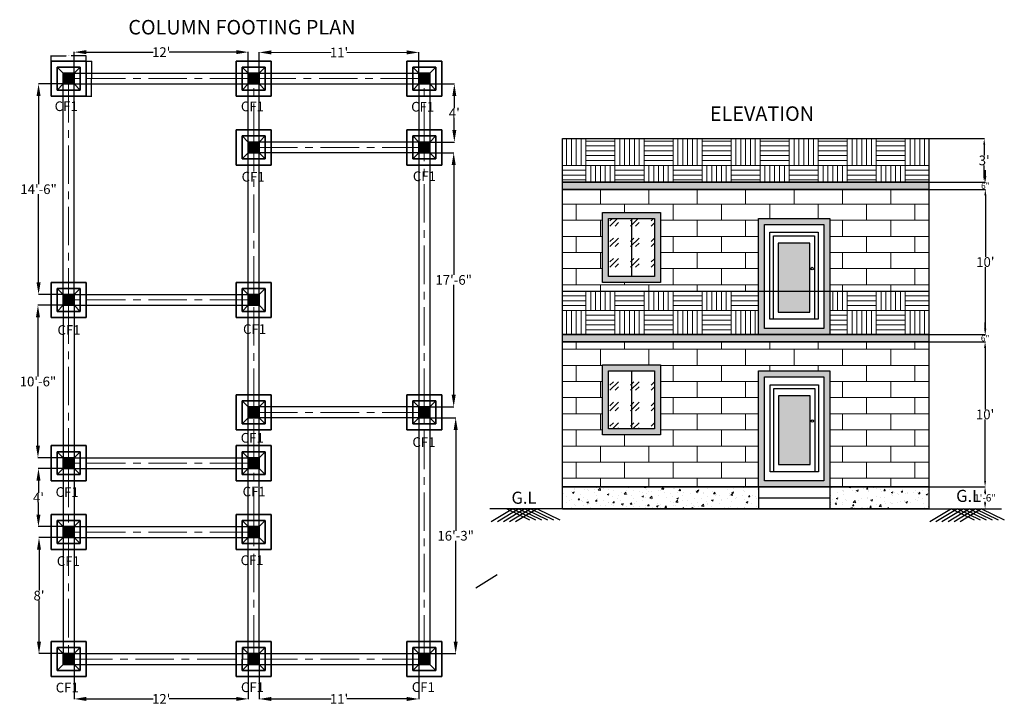
# Model space of a CAD drawing. Units: inches. Extents: x -25 to 789, y -921 to 230.
# Tile 1 of 5: x -25 to 789, y -921 to -354. Entities that reach past the tile are written whole.
import ezdxf

# ---------------------------------------------------------------- set-up
doc = ezdxf.new("R2010")
doc.units = ezdxf.units.IN
doc.header["$MEASUREMENT"] = 0
doc.linetypes.add('CENTER', pattern=[50.8, 31.75, -6.35, 6.35, -6.35])
for name, color, linetype, lineweight in [('A-ANNO-DIMS', 2, 'Continuous', 18), ('A-ANNO-TEXT', 7, 'Continuous', 18), ('A-DOOR', 4, 'Continuous', 25), ('A-ELEV', 7, 'Continuous', 25), ('A-ELEV-PATT', 252, 'Continuous', 13), ('S-ANNO-DIMS', 2, 'Continuous', 18), ('S-ANNO-TEXT', 7, 'Continuous', 18), ('S-BEAM', 4, 'Continuous', 25), ('S-FNDN', 2, 'Continuous', 35), ('S-FNDN-PATT', 8, 'Continuous', 13), ('S-GRID', 6, 'CENTER', 18)]:
    doc.layers.add(name, color=color, linetype=linetype, lineweight=lineweight)
doc.styles.get("Standard").update_dxf_attribs({"font": 'arial.ttf'})
doc.dimstyles.get("Standard").update_dxf_attribs({"dimtxt": 0.18, "dimasz": 0.18, "dimexe": 0.18, "dimexo": 0.0625, "dimgap": 0.09, "dimtad": 0, "dimtih": 1, "dimtoh": 1, "dimdec": 1, "dimzin": 0, "dimdsep": 46, "dimlunit": 4, "dimtxsty": 'Standard', "dimcen": 0.09, "dimadec": 0, "dimazin": 0, "dimtfac": 1, "dimtdec": 1, "dimtofl": 0, "dimtmove": 0, "dimatfit": 3, "dimfxl": 1, "dimtolj": 1, "dimtzin": 0, "dimarcsym": 0})

# ---------------------------------------------------------------- blocks, each defined once
blk = doc.blocks.new('*U29')
blk.add_lwpolyline([(3.12, 0.01), (0.12, 0.01), (0.12, 72.01), (40.12, 72.01), (40.12, 0.01), (37.12, 0.01)])
for points in [[(37.12, 68.99), (37.12, 0.01), (3.12, 0.01), (3.12, 68.99)], [(33.12, 6.01), (33.12, 62.99), (7.12, 62.99), (7.12, 6.01)]]:
    blk.add_lwpolyline(points, close=True)
blk.add_circle((35.12, 42.01), 1)
blk = doc.blocks.new('*D30')
at = {"layer": 'A-ANNO-DIMS', "color": 0, "lineweight": -2, "transparency": 16777216}
for p, q in [((773.58, -483.04), (773.58, -478.04)), ((727.04, -488.04), (773.76, -488.04)), ((727.04, -494.04), (773.76, -494.04)), ((773.58, -499.04), (773.58, -504.04))]:
    blk.add_line(p, q, dxfattribs=at)
at = {"layer": 'A-ANNO-DIMS', "color": 0, "transparency": 16777216}
for points in [[(772.75, -483.04), (774.42, -483.04), (773.58, -488.04)], [(772.75, -499.04), (774.42, -499.04), (773.58, -494.04)]]:
    blk.add_solid(points, dxfattribs=at)
at = {"layer": 'Defpoints', "color": 0, "transparency": 16777216}
for p in [(726.98, -488.04), (773.58, -488.04), (726.98, -494.04)]:
    blk.add_point(p, dxfattribs=at)
at = {"layer": 'A-ANNO-DIMS', "color": 0, "transparency": 16777216, "insert": (773.58, -491.04), "char_height": 5, "attachment_point": 5}
blk.add_mtext('\\A1;6"', dxfattribs=at)
blk = doc.blocks.new('*D31')
at = {"layer": 'A-ANNO-DIMS', "color": 0, "lineweight": -2, "transparency": 16777216}
for p, q in [((727.04, -452.04), (772.82, -452.04)), ((772.64, -457.04), (772.64, -465.87)), ((772.64, -483.04), (772.64, -474.22)), ((727.04, -488.04), (772.82, -488.04))]:
    blk.add_line(p, q, dxfattribs=at)
at = {"layer": 'A-ANNO-DIMS', "color": 0, "transparency": 16777216}
for points in [[(771.81, -457.04), (773.48, -457.04), (772.64, -452.04)], [(771.81, -483.04), (773.48, -483.04), (772.64, -488.04)]]:
    blk.add_solid(points, dxfattribs=at)
at = {"layer": 'Defpoints', "color": 0, "transparency": 16777216}
for p in [(726.98, -452.04), (772.64, -452.04), (726.98, -488.04)]:
    blk.add_point(p, dxfattribs=at)
at = {"layer": 'A-ANNO-DIMS', "color": 0, "transparency": 16777216, "insert": (772.64, -470.04), "char_height": 8, "attachment_point": 5}
blk.add_mtext("\\A1;3'", dxfattribs=at)
blk = doc.blocks.new('*D32')
at = {"layer": 'A-ANNO-DIMS', "color": 0, "lineweight": -2, "transparency": 16777216}
for p, q in [((727.04, -740.04), (773.55, -740.04)), ((773.37, -745.04), (773.37, -745.89)), ((773.37, -753.04), (773.37, -752.2)), ((727.04, -758.04), (773.55, -758.04))]:
    blk.add_line(p, q, dxfattribs=at)
at = {"layer": 'A-ANNO-DIMS', "color": 0, "transparency": 16777216}
for points in [[(772.53, -745.04), (774.2, -745.04), (773.37, -740.04)], [(772.53, -753.04), (774.2, -753.04), (773.37, -758.04)]]:
    blk.add_solid(points, dxfattribs=at)
at = {"layer": 'Defpoints', "color": 0, "transparency": 16777216}
for p in [(726.98, -740.04), (773.37, -740.04), (726.98, -758.04)]:
    blk.add_point(p, dxfattribs=at)
at = {"layer": 'A-ANNO-DIMS', "color": 0, "transparency": 16777216, "insert": (773.37, -749.04), "char_height": 6, "attachment_point": 5}
blk.add_mtext('\\A1;1\'-6"', dxfattribs=at)
blk = doc.blocks.new('*D33')
at = {"layer": 'A-ANNO-DIMS', "color": 0, "lineweight": -2, "transparency": 16777216}
for p, q in [((727.04, -620.04), (773.55, -620.04)), ((773.37, -625.04), (773.37, -675.87)), ((773.37, -735.04), (773.37, -684.22)), ((727.04, -740.04), (773.55, -740.04))]:
    blk.add_line(p, q, dxfattribs=at)
at = {"layer": 'A-ANNO-DIMS', "color": 0, "transparency": 16777216}
for points in [[(772.54, -625.04), (774.2, -625.04), (773.37, -620.04)], [(772.54, -735.04), (774.2, -735.04), (773.37, -740.04)]]:
    blk.add_solid(points, dxfattribs=at)
at = {"layer": 'Defpoints', "color": 0, "transparency": 16777216}
for p in [(726.98, -620.04), (773.37, -620.04), (726.98, -740.04)]:
    blk.add_point(p, dxfattribs=at)
at = {"layer": 'A-ANNO-DIMS', "color": 0, "transparency": 16777216, "insert": (773.37, -680.04), "char_height": 8, "attachment_point": 5}
blk.add_mtext("\\A1;10'", dxfattribs=at)
blk = doc.blocks.new('*D34')
at = {"layer": 'A-ANNO-DIMS', "color": 0, "lineweight": -2, "transparency": 16777216}
for p, q in [((773.4, -609.04), (773.4, -604.04)), ((727.04, -614.04), (773.58, -614.04)), ((727.04, -620.04), (773.58, -620.04)), ((773.4, -625.04), (773.4, -630.04))]:
    blk.add_line(p, q, dxfattribs=at)
at = {"layer": 'A-ANNO-DIMS', "color": 0, "transparency": 16777216}
for points in [[(772.57, -609.04), (774.24, -609.04), (773.4, -614.04)], [(772.57, -625.04), (774.24, -625.04), (773.4, -620.04)]]:
    blk.add_solid(points, dxfattribs=at)
at = {"layer": 'Defpoints', "color": 0, "transparency": 16777216}
for p in [(726.98, -614.04), (773.4, -614.04), (726.98, -620.04)]:
    blk.add_point(p, dxfattribs=at)
at = {"layer": 'A-ANNO-DIMS', "color": 0, "transparency": 16777216, "insert": (773.4, -617.04), "char_height": 5, "attachment_point": 5}
blk.add_mtext('\\A1;6"', dxfattribs=at)
blk = doc.blocks.new('*D35')
at = {"layer": 'A-ANNO-DIMS', "color": 0, "lineweight": -2, "transparency": 16777216}
for p, q in [((727.04, -494.04), (773.76, -494.04)), ((773.58, -499.04), (773.58, -549.87)), ((773.58, -609.04), (773.58, -558.22)), ((727.04, -614.04), (773.76, -614.04))]:
    blk.add_line(p, q, dxfattribs=at)
at = {"layer": 'A-ANNO-DIMS', "color": 0, "transparency": 16777216}
for points in [[(772.75, -499.04), (774.42, -499.04), (773.58, -494.04)], [(772.75, -609.04), (774.42, -609.04), (773.58, -614.04)]]:
    blk.add_solid(points, dxfattribs=at)
at = {"layer": 'Defpoints', "color": 0, "transparency": 16777216}
for p in [(726.98, -494.04), (726.98, -614.04), (773.58, -614.04)]:
    blk.add_point(p, dxfattribs=at)
at = {"layer": 'A-ANNO-DIMS', "color": 0, "transparency": 16777216, "insert": (773.58, -554.04), "char_height": 8, "attachment_point": 5}
blk.add_mtext("\\A1;10'", dxfattribs=at)
blk = doc.blocks.new('*D36')
at = {"layer": 'Defpoints', "color": 0, "transparency": 16777216}
for p in [(173.31, -877.85), (305.31, -877.85), (305.31, -915.32)]:
    blk.add_point(p, dxfattribs=at)
at = {"layer": 'S-ANNO-DIMS', "color": 0, "lineweight": -2, "transparency": 16777216}
for p, q in [((173.31, -877.91), (173.31, -915.5)), ((305.31, -877.91), (305.31, -915.5)), ((183.31, -915.32), (232.81, -915.32)), ((295.31, -915.32), (245.82, -915.32))]:
    blk.add_line(p, q, dxfattribs=at)
at = {"layer": 'S-ANNO-DIMS', "color": 0, "transparency": 16777216}
for points in [[(183.31, -913.65), (183.31, -916.98), (173.31, -915.32)], [(295.31, -913.65), (295.31, -916.98), (305.31, -915.32)]]:
    blk.add_solid(points, dxfattribs=at)
at = {"layer": 'S-ANNO-DIMS', "color": 0, "transparency": 16777216, "insert": (239.31, -915.32), "char_height": 8, "attachment_point": 5}
blk.add_mtext("\\A1;11'", dxfattribs=at)
blk = doc.blocks.new('*D37')
at = {"layer": 'Defpoints', "color": 0, "transparency": 16777216}
for p in [(20.31, -877.85), (164.31, -877.85), (164.31, -915.27)]:
    blk.add_point(p, dxfattribs=at)
at = {"layer": 'S-ANNO-DIMS', "color": 0, "lineweight": -2, "transparency": 16777216}
for p, q in [((20.31, -877.91), (20.31, -915.45)), ((164.31, -877.91), (164.31, -915.45)), ((30.31, -915.27), (85.81, -915.27)), ((154.31, -915.27), (98.82, -915.27))]:
    blk.add_line(p, q, dxfattribs=at)
at = {"layer": 'S-ANNO-DIMS', "color": 0, "transparency": 16777216}
for points in [[(30.31, -913.61), (30.31, -916.94), (20.31, -915.27)], [(154.31, -913.61), (154.31, -916.94), (164.31, -915.27)]]:
    blk.add_solid(points, dxfattribs=at)
at = {"layer": 'S-ANNO-DIMS', "color": 0, "transparency": 16777216, "insert": (92.31, -915.27), "char_height": 8, "attachment_point": 5}
blk.add_mtext("\\A1;12'", dxfattribs=at)
blk = doc.blocks.new('*D38')
at = {"layer": 'Defpoints', "color": 0, "transparency": 16777216}
for p in [(305.31, -682.85), (335.74, -682.85), (305.31, -877.85)]:
    blk.add_point(p, dxfattribs=at)
at = {"layer": 'S-ANNO-DIMS', "color": 0, "lineweight": -2, "transparency": 16777216}
for p, q in [((305.38, -682.85), (335.92, -682.85)), ((335.74, -692.85), (335.74, -776.17)), ((335.74, -867.85), (335.74, -784.52)), ((305.38, -877.85), (335.92, -877.85))]:
    blk.add_line(p, q, dxfattribs=at)
at = {"layer": 'S-ANNO-DIMS', "color": 0, "transparency": 16777216}
for points in [[(334.08, -692.85), (337.41, -692.85), (335.74, -682.85)], [(334.08, -867.85), (337.41, -867.85), (335.74, -877.85)]]:
    blk.add_solid(points, dxfattribs=at)
at = {"layer": 'S-ANNO-DIMS', "color": 0, "transparency": 16777216, "insert": (335.74, -780.35), "char_height": 8, "attachment_point": 5}
blk.add_mtext('\\A1;16\'-3"', dxfattribs=at)
blk = doc.blocks.new('*D39')
at = {"layer": 'Defpoints', "color": 0, "transparency": 16777216}
for p in [(305.31, -463.85), (334.1, -463.85), (305.31, -673.85)]:
    blk.add_point(p, dxfattribs=at)
at = {"layer": 'S-ANNO-DIMS', "color": 0, "lineweight": -2, "transparency": 16777216}
for p, q in [((305.38, -463.85), (334.28, -463.85)), ((334.1, -473.85), (334.1, -564.67)), ((334.1, -663.85), (334.1, -573.02)), ((305.38, -673.85), (334.28, -673.85))]:
    blk.add_line(p, q, dxfattribs=at)
at = {"layer": 'S-ANNO-DIMS', "color": 0, "transparency": 16777216}
for points in [[(332.44, -473.85), (335.77, -473.85), (334.1, -463.85)], [(332.44, -663.85), (335.77, -663.85), (334.1, -673.85)]]:
    blk.add_solid(points, dxfattribs=at)
at = {"layer": 'S-ANNO-DIMS', "color": 0, "transparency": 16777216, "insert": (334.1, -568.85), "char_height": 8, "attachment_point": 5}
blk.add_mtext('\\A1;17\'-6"', dxfattribs=at)
blk = doc.blocks.new('*D40')
at = {"layer": 'Defpoints', "color": 0, "transparency": 16777216}
for p in [(305.31, -406.85), (305.31, -454.85), (334.62, -454.85)]:
    blk.add_point(p, dxfattribs=at)
at = {"layer": 'S-ANNO-DIMS', "color": 0, "lineweight": -2, "transparency": 16777216}
for p, q in [((305.38, -406.85), (334.8, -406.85)), ((334.62, -416.85), (334.62, -426.76)), ((334.62, -444.85), (334.62, -434.94)), ((305.38, -454.85), (334.8, -454.85))]:
    blk.add_line(p, q, dxfattribs=at)
at = {"layer": 'S-ANNO-DIMS', "color": 0, "transparency": 16777216}
for points in [[(332.96, -416.85), (336.29, -416.85), (334.62, -406.85)], [(332.96, -444.85), (336.29, -444.85), (334.62, -454.85)]]:
    blk.add_solid(points, dxfattribs=at)
at = {"layer": 'S-ANNO-DIMS', "color": 0, "transparency": 16777216, "insert": (334.62, -430.85), "char_height": 8, "attachment_point": 5}
blk.add_mtext("\\A1;4'", dxfattribs=at)
blk = doc.blocks.new('*D41')
at = {"layer": 'Defpoints', "color": 0, "transparency": 16777216}
for p in [(305.31, -380.75), (173.31, -406.85), (305.31, -406.85)]:
    blk.add_point(p, dxfattribs=at)
at = {"layer": 'S-ANNO-DIMS', "color": 0, "lineweight": -2, "transparency": 16777216}
for p, q in [((173.31, -406.78), (173.31, -380.57)), ((305.31, -406.78), (305.31, -380.57))]:
    blk.add_line(p, q, dxfattribs=at)
at = {"layer": 'S-ANNO-DIMS', "color": 0, "lineweight": 9, "transparency": 16777216}
for p, q in [((183.31, -380.75), (232.81, -380.75)), ((295.31, -380.75), (245.82, -380.75))]:
    blk.add_line(p, q, dxfattribs=at)
at = {"layer": 'S-ANNO-DIMS', "color": 0, "transparency": 16777216}
for points in [[(183.31, -379.09), (183.31, -382.42), (173.31, -380.75)], [(295.31, -379.09), (295.31, -382.42), (305.31, -380.75)]]:
    blk.add_solid(points, dxfattribs=at)
at = {"layer": 'S-ANNO-DIMS', "color": 0, "transparency": 16777216, "insert": (239.31, -380.75), "char_height": 8, "attachment_point": 5}
blk.add_mtext("\\A1;11'", dxfattribs=at)
blk = doc.blocks.new('*D42')
at = {"layer": 'Defpoints', "color": 0, "transparency": 16777216}
for p in [(164.31, -380.51), (20.31, -406.85), (164.31, -406.85)]:
    blk.add_point(p, dxfattribs=at)
at = {"layer": 'S-ANNO-DIMS', "color": 0, "lineweight": -2, "transparency": 16777216}
for p, q in [((20.31, -406.78), (20.31, -380.33)), ((30.31, -380.51), (85.81, -380.51)), ((154.31, -380.51), (98.82, -380.51)), ((164.31, -406.78), (164.31, -380.33))]:
    blk.add_line(p, q, dxfattribs=at)
at = {"layer": 'S-ANNO-DIMS', "color": 0, "transparency": 16777216}
for points in [[(30.31, -378.84), (30.31, -382.18), (20.31, -380.51)], [(154.31, -378.84), (154.31, -382.18), (164.31, -380.51)]]:
    blk.add_solid(points, dxfattribs=at)
at = {"layer": 'S-ANNO-DIMS', "color": 0, "transparency": 16777216, "insert": (92.31, -380.51), "char_height": 8, "attachment_point": 5}
blk.add_mtext("\\A1;12'", dxfattribs=at)
blk = doc.blocks.new('*D43')
at = {"layer": 'Defpoints', "color": 0, "transparency": 16777216}
for p in [(20.31, -406.85), (-9.06, -580.85), (20.31, -580.85)]:
    blk.add_point(p, dxfattribs=at)
at = {"layer": 'S-ANNO-DIMS', "color": 0, "lineweight": -2, "transparency": 16777216}
for p, q in [((20.25, -406.85), (-9.24, -406.85)), ((-9.06, -416.85), (-9.06, -489.67)), ((-9.06, -570.85), (-9.06, -498.02)), ((20.25, -580.85), (-9.24, -580.85))]:
    blk.add_line(p, q, dxfattribs=at)
at = {"layer": 'S-ANNO-DIMS', "color": 0, "transparency": 16777216}
for points in [[(-10.73, -416.85), (-7.39, -416.85), (-9.06, -406.85)], [(-10.73, -570.85), (-7.39, -570.85), (-9.06, -580.85)]]:
    blk.add_solid(points, dxfattribs=at)
at = {"layer": 'S-ANNO-DIMS', "color": 0, "transparency": 16777216, "insert": (-9.06, -493.85), "char_height": 8, "attachment_point": 5}
blk.add_mtext('\\A1;14\'-6"', dxfattribs=at)
blk = doc.blocks.new('*D44')
at = {"layer": 'Defpoints', "color": 0, "transparency": 16777216}
for p in [(20.31, -589.85), (-9.58, -715.85), (20.31, -715.85)]:
    blk.add_point(p, dxfattribs=at)
at = {"layer": 'S-ANNO-DIMS', "color": 0, "lineweight": -2, "transparency": 16777216}
for p, q in [((20.25, -589.85), (-9.76, -589.85)), ((-9.58, -599.85), (-9.58, -648.67)), ((-9.58, -705.85), (-9.58, -657.02)), ((20.25, -715.85), (-9.76, -715.85))]:
    blk.add_line(p, q, dxfattribs=at)
at = {"layer": 'S-ANNO-DIMS', "color": 0, "transparency": 16777216}
for points in [[(-11.24, -599.85), (-7.91, -599.85), (-9.58, -589.85)], [(-11.24, -705.85), (-7.91, -705.85), (-9.58, -715.85)]]:
    blk.add_solid(points, dxfattribs=at)
at = {"layer": 'S-ANNO-DIMS', "color": 0, "transparency": 16777216, "insert": (-9.58, -652.85), "char_height": 8, "attachment_point": 5}
blk.add_mtext('\\A1;10\'-6"', dxfattribs=at)
blk = doc.blocks.new('*D45')
at = {"layer": 'Defpoints', "color": 0, "transparency": 16777216}
for p in [(20.31, -724.85), (-9.14, -772.85), (20.31, -772.85)]:
    blk.add_point(p, dxfattribs=at)
at = {"layer": 'S-ANNO-DIMS', "color": 0, "lineweight": -2, "transparency": 16777216}
for p, q in [((20.25, -724.85), (-9.32, -724.85)), ((-9.14, -734.85), (-9.14, -744.76)), ((-9.14, -762.85), (-9.14, -752.94)), ((20.25, -772.85), (-9.32, -772.85))]:
    blk.add_line(p, q, dxfattribs=at)
at = {"layer": 'S-ANNO-DIMS', "color": 0, "transparency": 16777216}
for points in [[(-10.81, -734.85), (-7.47, -734.85), (-9.14, -724.85)], [(-10.81, -762.85), (-7.47, -762.85), (-9.14, -772.85)]]:
    blk.add_solid(points, dxfattribs=at)
at = {"layer": 'S-ANNO-DIMS', "color": 0, "transparency": 16777216, "insert": (-9.14, -748.85), "char_height": 8, "attachment_point": 5}
blk.add_mtext("\\A1;4'", dxfattribs=at)
blk = doc.blocks.new('*D46')
at = {"layer": 'Defpoints', "color": 0, "transparency": 16777216}
for p in [(-8.7, -781.85), (20.31, -781.85), (20.31, -877.85)]:
    blk.add_point(p, dxfattribs=at)
at = {"layer": 'S-ANNO-DIMS', "color": 0, "lineweight": -2, "transparency": 16777216}
for p, q in [((20.25, -781.85), (-8.88, -781.85)), ((-8.7, -791.85), (-8.7, -825.67)), ((-8.7, -867.85), (-8.7, -834.02)), ((20.25, -877.85), (-8.88, -877.85))]:
    blk.add_line(p, q, dxfattribs=at)
at = {"layer": 'S-ANNO-DIMS', "color": 0, "transparency": 16777216}
for points in [[(-10.36, -791.85), (-7.03, -791.85), (-8.7, -781.85)], [(-10.36, -867.85), (-7.03, -867.85), (-8.7, -877.85)]]:
    blk.add_solid(points, dxfattribs=at)
at = {"layer": 'S-ANNO-DIMS', "color": 0, "transparency": 16777216, "insert": (-8.7, -829.85), "char_height": 8, "attachment_point": 5}
blk.add_mtext("\\A1;8'", dxfattribs=at)
blk = doc.blocks.new('FOOTING-CF1')
at = {"ltscale": 0.5}
for p, q in [((0, 29), (29, 29)), ((0, 0), (0, 29)), ((29, 29), (29, 0)), ((29, 0), (0, 0))]:
    blk.add_line(p, q, dxfattribs=at)
for p, q in [((5, 24), (10, 19)), ((5, 5), (5, 24)), ((5, 24), (24, 24)), ((10, 10), (10, 19)), ((10, 19), (19, 19)), ((24, 24), (19, 19)), ((19, 19), (19, 10)), ((24, 24), (24, 5)), ((10, 10), (5, 5)), ((19, 10), (10, 10)), ((19, 10), (24, 5)), ((24, 5), (5, 5))]:
    blk.add_line(p, q)
blk = doc.blocks.new('GL-EARTH-SYMB')
for q in [(0, 0), (36.54, 1.75)]:
    blk.add_line((17.79, 10.92), q)
blk = doc.blocks.new('*D79')
at = {"layer": 'A-ANNO-DIMS', "color": 0, "lineweight": -2, "transparency": 16777216}
for p, q in [((1.31, -387.78), (1.31, -383.32)), ((1.49, -383.5), (13.72, -383.5)), ((30.13, -383.5), (17.91, -383.5)), ((30.31, -387.78), (30.31, -383.32))]:
    blk.add_line(p, q, dxfattribs=at)
at = {"layer": 'A-ANNO-DIMS', "color": 0, "transparency": 16777216}
for points in [[(1.49, -383.47), (1.49, -383.53), (1.31, -383.5)], [(30.13, -383.47), (30.13, -383.53), (30.31, -383.5)]]:
    blk.add_solid(points, dxfattribs=at)
at = {"layer": 'Defpoints', "color": 0, "transparency": 16777216}
for p in [(1.31, -383.5), (1.31, -387.85), (30.31, -387.85)]:
    blk.add_point(p, dxfattribs=at)
at = {"layer": 'A-ANNO-DIMS', "color": 0, "transparency": 16777216, "insert": (15.81, -383.5), "char_height": 0.18, "attachment_point": 5}
blk.add_mtext('\\A1;COLUMN FOOTING CF1 2\'-5" TYP.', dxfattribs=at)
blk = doc.blocks.new('*D80')
at = {"layer": 'A-ANNO-DIMS', "color": 0, "lineweight": -2, "transparency": 16777216}
for p, q in [((30.38, -387.85), (34.84, -387.85)), ((34.66, -388.03), (34.66, -402.16)), ((34.66, -416.67), (34.66, -402.53)), ((30.38, -416.85), (34.84, -416.85))]:
    blk.add_line(p, q, dxfattribs=at)
at = {"layer": 'A-ANNO-DIMS', "color": 0, "transparency": 16777216}
for points in [[(34.63, -388.03), (34.69, -388.03), (34.66, -387.85)], [(34.63, -416.67), (34.69, -416.67), (34.66, -416.85)]]:
    blk.add_solid(points, dxfattribs=at)
at = {"layer": 'Defpoints', "color": 0, "transparency": 16777216}
for p in [(30.31, -387.85), (34.66, -387.85), (30.31, -416.85)]:
    blk.add_point(p, dxfattribs=at)
at = {"layer": 'A-ANNO-DIMS', "color": 0, "transparency": 16777216, "insert": (34.66, -402.35), "char_height": 0.18, "attachment_point": 5}
blk.add_mtext('\\A1;2\'-5" TYP.', dxfattribs=at)

msp = doc.modelspace()

# ---------------------------------------------------------------- hatches: boundary and pattern name
at = {"layer": 'A-ELEV-PATT'}
h = msp.add_hatch(dxfattribs=at)
h.set_pattern_fill('AR-PARQ1', color=256, scale=2)
h.set_pattern_definition([(90, (395.404, -66.132), (-24, 24), [24, -24]), (90, (399.404, -66.132), (-24, 24), [24, -24]), (90, (403.404, -66.132), (-24, 24), [24, -24]), (90, (407.404, -66.132), (-24, 24), [24, -24]), (90, (411.404, -66.132), (-24, 24), [24, -24]), (90, (415.404, -66.132), (-24, 24), [24, -24]), (90, (419.404, -66.132), (-24, 24), [24, -24]), (0, (395.404, -42.132), (24, -24), [24, -24]), (0, (395.404, -38.132), (24, -24), [24, -24]), (0, (395.404, -34.132), (24, -24), [24, -24]), (0, (395.404, -30.132), (24, -24), [24, -24]), (0, (395.404, -26.132), (24, -24), [24, -24]), (0, (395.404, -22.132), (24, -24), [24, -24]), (0, (395.404, -18.132), (24, -24), [24, -24])])
h.paths.add_polyline_path([(585.98, -578.04), (423.98, -578.04), (423.98, -614.04), (585.98, -614.04)])
h.paths.add_polyline_path([(726.98, -578.04), (645.04, -578.04), (645.04, -614.04), (726.98, -614.04)])
h.paths.add_polyline_path([(726.98, -452.04), (423.98, -452.04), (423.98, -488.04), (726.98, -488.04)])
h = msp.add_hatch(color=256, dxfattribs=at)
h.dxf.hatch_style = 1
h.paths.add_polyline_path([(423.98, -614.04), (423.98, -620.04), (726.98, -620.04), (726.98, -614.04)])
h.paths.add_polyline_path([(423.98, -488.04), (423.98, -494.04), (726.98, -494.04), (726.98, -488.04)])
h = msp.add_hatch(dxfattribs=at)
h.set_pattern_fill('AR-BRSTD', color=256, scale=5)
h.set_pattern_definition([(0, (395.404, -66.132), (0, 13.335), []), (90, (395.404, -66.132), (-20, 13.335), [13.335, -13.335])])
h.paths.add_polyline_path([(585.98, -644.04), (645.04, -644.04), (645.04, -740.04), (726.98, -740.04), (726.98, -620.04), (423.98, -620.04), (423.98, -740.04), (585.98, -740.04)])
h.paths.add_polyline_path([(504.98, -697.04), (456.98, -697.04), (456.98, -639.04), (504.98, -639.04)], flags=16)
h.paths.add_polyline_path([(499.98, -692.04), (461.98, -692.04), (461.98, -644.04), (499.98, -644.04)], flags=0)
h.paths.add_polyline_path([(585.98, -518.04), (645.04, -518.04), (645.04, -578.04), (726.98, -578.04), (726.98, -494.04), (423.98, -494.04), (423.98, -578.04), (585.98, -578.04)])
h.paths.add_polyline_path([(504.98, -571.04), (456.98, -571.04), (456.98, -513.04), (504.98, -513.04)], flags=16)
h.paths.add_polyline_path([(499.98, -566.04), (461.98, -566.04), (461.98, -518.04), (499.98, -518.04)], flags=0)
h = msp.add_hatch(color=256, dxfattribs=at)
h.dxf.hatch_style = 1
h.paths.add_polyline_path([(504.98, -639.04), (456.98, -639.04), (456.98, -697.04), (504.98, -697.04)])
h.paths.add_polyline_path([(461.98, -692.04), (461.98, -644.04), (499.98, -644.04), (499.98, -692.04)], flags=16)
h.paths.add_polyline_path([(645.04, -644.04), (585.98, -644.04), (585.98, -740.04), (645.04, -740.04)])
h.paths.add_polyline_path([(590.98, -649.04), (640.04, -649.04), (640.04, -735.04), (590.98, -735.04)], flags=16)
h.paths.add_polyline_path([(504.98, -513.04), (456.98, -513.04), (456.98, -571.04), (504.98, -571.04)])
h.paths.add_polyline_path([(461.98, -566.04), (461.98, -518.04), (499.98, -518.04), (499.98, -566.04)], flags=16)
h.paths.add_polyline_path([(590.98, -578.04), (585.98, -578.04), (585.98, -614.04), (645.04, -614.04), (645.04, -578.04), (640.04, -578.04), (640.04, -609.04), (590.98, -609.04)])
h.paths.add_polyline_path([(590.98, -523.04), (640.04, -523.04), (640.04, -578.04), (645.04, -578.04), (645.04, -518.04), (585.98, -518.04), (585.98, -578.04), (590.98, -578.04)])
h = msp.add_hatch(dxfattribs=at)
h.set_pattern_fill('GOST_GLASS', color=256, scale=2)
h.set_pattern_definition([(45, (395.404, -66.132), (16.97056, -2e-15), [10, -14]), (45, (399.647, -66.132), (16.97056, -2e-15), [4, -20]), (45, (395.404, -61.89), (16.97056, -2e-15), [4, -20])])
h.paths.add_polyline_path([(480.98, -518.04), (461.98, -518.04), (461.98, -566.04), (480.98, -566.04)])
h.paths.add_polyline_path([(499.98, -518.04), (480.98, -518.04), (480.98, -566.04), (499.98, -566.04)])
h.paths.add_polyline_path([(480.98, -644.04), (461.98, -644.04), (461.98, -692.04), (480.98, -692.04)])
h.paths.add_polyline_path([(499.98, -644.04), (480.98, -644.04), (480.98, -692.04), (499.98, -692.04)])
h = msp.add_hatch(color=256, dxfattribs=at)
h.dxf.hatch_style = 1
h.paths.add_polyline_path([(628.41, -538.45), (602.41, -538.45), (602.41, -578.04), (628.41, -578.04)])
h.paths.add_polyline_path([(628.41, -578.04), (602.41, -578.04), (602.41, -595.43), (628.41, -595.43)])
h.paths.add_polyline_path([(628.65, -664.6), (602.65, -664.6), (602.65, -721.58), (628.65, -721.58)])
h = msp.add_hatch(dxfattribs=at)
h.set_pattern_fill('AR-CONC', color=256, scale=2)
h.set_pattern_definition([(50, (395.404, -66.132), (14.3452, -1.25504), [1.5, -16.5]), (355, (395.404, -66.132), (-2.77503, 15.04384), [1.2, -13.2]), (100.4514, (396.6, -66.237), (11.57018, 13.7888), [1.2748, -14.02284]), (46.1842, (395.404, -62.132), (21.34483, -3.3104), [2.25, -24.75]), (96.6356, (397.183, -62.408), (18.69324, 19.4824), [1.9122, -21.0343]), (351.184, (395.404, -62.132), (18.69324, 19.4824), [1.8, -19.8]), (21, (397.404, -63.132), (11.93814, -8.05238), [1.5, -16.5]), (326, (397.404, -63.132), (4.8663, 14.503), [1.2, -13.2]), (71.4514, (398.399, -63.803), (16.80445, 6.45062), [1.2748, -14.02284]), (37.5, (395.404, -66.132), (0.243197, 6.657877), [0, -13.04, 0, -13.4, 0, -13.25]), (7.5, (395.404, -66.132), (5.26139, 7.888234), [0, -7.64, 0, -12.74, 0, -5.05]), (327.5, (390.944, -66.132), (10.67645, -0.451097), [0, -5, 0, -15.6, 0, -20.7]), (317.5, (388.944, -66.132), (11.66372, 2.0021), [0, -6.5, 0, -10.36, 0, -14.7])])
h.paths.add_polyline_path([(423.98, -740.04), (423.98, -758.04), (585.98, -758.04), (585.98, -740.04)])
h.paths.add_polyline_path([(645.04, -740.04), (645.04, -758.04), (726.98, -758.04), (726.98, -740.04)])
at = {"layer": 'S-FNDN-PATT'}
h = msp.add_hatch(dxfattribs=at)
h.set_pattern_fill('ANSI31', color=256)
h.set_pattern_definition([(45, (377.53263, -562.60124), (-0.088388348, 0.088388348), [])])
h.paths.add_polyline_path([(20.31, -397.85), (11.31, -397.85), (11.31, -406.85), (20.31, -406.85)])
h.paths.add_polyline_path([(164.31, -406.85), (173.31, -406.85), (173.31, -397.85), (164.31, -397.85)])
h.paths.add_polyline_path([(314.31, -397.85), (305.31, -397.85), (305.31, -406.85), (314.31, -406.85)])
h.paths.add_polyline_path([(173.31, -454.85), (164.31, -454.85), (164.31, -463.85), (173.31, -463.85)])
h.paths.add_polyline_path([(314.31, -454.85), (305.31, -454.85), (305.31, -463.85), (314.31, -463.85)])
h.paths.add_polyline_path([(164.31, -589.85), (173.31, -589.85), (173.31, -580.85), (164.31, -580.85)])
h.paths.add_polyline_path([(20.31, -580.85), (11.31, -580.85), (11.31, -589.85), (20.31, -589.85)])
h.paths.add_polyline_path([(164.31, -682.85), (173.31, -682.85), (173.31, -673.85), (164.31, -673.85)])
h.paths.add_polyline_path([(305.31, -682.85), (314.31, -682.85), (314.31, -673.85), (305.31, -673.85)])
h.paths.add_polyline_path([(11.31, -715.85), (11.31, -724.85), (20.31, -724.85), (20.31, -715.85)])
h.paths.add_polyline_path([(164.31, -715.85), (164.31, -724.85), (173.31, -724.85), (173.31, -715.85)])
h.paths.add_polyline_path([(11.31, -781.85), (20.31, -781.85), (20.31, -772.85), (11.31, -772.85)])
h.paths.add_polyline_path([(164.31, -781.85), (173.31, -781.85), (173.31, -772.85), (164.31, -772.85)])
h.paths.add_polyline_path([(11.31, -877.85), (11.31, -886.85), (20.31, -886.85), (20.31, -877.85)])
h.paths.add_polyline_path([(164.31, -886.85), (173.31, -886.85), (173.31, -877.85), (164.31, -877.85)])
h.paths.add_polyline_path([(314.31, -877.85), (305.31, -877.85), (305.31, -886.85), (314.31, -886.85)])

# ---------------------------------------------------------------- linework, layer by layer
at = {"layer": 'A-ELEV'}
for p, q in [((423.98, -452.04), (726.98, -452.04)), ((423.98, -488.04), (726.98, -488.04)), ((423.98, -494.04), (726.98, -494.04)), ((480.98, -518.04), (480.98, -566.04)), ((423.98, -578.04), (726.98, -578.04)), ((423.98, -614.04), (726.98, -614.04)), ((423.98, -614.04), (726.98, -614.04)), ((423.98, -620.04), (726.98, -620.04)), ((480.98, -644.04), (480.98, -692.04)), ((423.98, -740.04), (726.98, -740.04)), ((585.98, -740.04), (645.04, -740.04)), ((585.98, -740.04), (585.98, -758.04)), ((645.04, -740.04), (645.04, -758.04)), ((585.98, -749.04), (645.04, -749.04)), ((423.98, -758.04), (363.98, -758.04)), ((377.97, -758.04), (396.72, -767.22)), ((423.98, -758.04), (726.98, -758.04)), ((726.98, -758.04), (786.98, -758.04)), ((370.14, -812.8), (352.35, -823.73))]:
    msp.add_line(p, q, dxfattribs=at)
for points in [[(423.98, -452.04), (726.98, -452.04), (726.98, -488.04), (423.98, -488.04)], [(423.98, -488.04), (726.98, -488.04), (726.98, -494.04), (423.98, -494.04)], [(423.98, -494.04), (726.98, -494.04), (726.98, -614.04), (423.98, -614.04)], [(456.98, -513.04), (504.98, -513.04), (504.98, -571.04), (456.98, -571.04)], [(461.98, -518.04), (499.98, -518.04), (499.98, -566.04), (461.98, -566.04)], [(585.98, -518.04), (645.04, -518.04), (645.04, -614.04), (585.98, -614.04)], [(590.98, -523.04), (640.04, -523.04), (640.04, -609.04), (590.98, -609.04)], [(423.98, -578.04), (726.98, -578.04), (726.98, -614.04), (423.98, -614.04)], [(423.98, -614.04), (726.98, -614.04), (726.98, -620.04), (423.98, -620.04)], [(423.98, -620.04), (726.98, -620.04), (726.98, -740.04), (423.98, -740.04)], [(456.98, -639.04), (504.98, -639.04), (504.98, -697.04), (456.98, -697.04)], [(461.98, -644.04), (499.98, -644.04), (499.98, -692.04), (461.98, -692.04)], [(585.98, -644.04), (645.04, -644.04), (645.04, -740.04), (585.98, -740.04)], [(590.98, -649.04), (640.04, -649.04), (640.04, -735.04), (590.98, -735.04)], [(423.98, -740.04), (726.98, -740.04), (726.98, -758.04), (423.98, -758.04)]]:
    msp.add_lwpolyline(points, close=True, dxfattribs=at)
at = {"layer": 'S-BEAM'}
for p, q in [((11.31, -589.85), (11.31, -397.85)), ((20.31, -397.85), (173.31, -397.85)), ((173.31, -397.85), (314.31, -397.85)), ((314.31, -397.85), (314.31, -463.85)), ((20.31, -580.85), (20.31, -406.85)), ((20.31, -406.85), (164.31, -406.85)), ((164.31, -454.85), (164.31, -406.85)), ((173.31, -454.85), (173.31, -406.85)), ((173.31, -406.85), (305.31, -406.85)), ((305.31, -406.85), (305.31, -454.85)), ((305.31, -454.85), (173.31, -454.85)), ((164.31, -580.85), (164.31, -463.85)), ((173.31, -589.85), (173.31, -463.85)), ((305.31, -463.85), (173.31, -463.85)), ((305.31, -463.85), (305.31, -673.85)), ((305.31, -463.85), (305.31, -886.85)), ((314.31, -463.85), (314.31, -886.85)), ((20.31, -580.85), (164.31, -580.85)), ((11.31, -589.85), (11.31, -724.85)), ((20.31, -589.85), (164.31, -589.85)), ((20.31, -589.85), (20.31, -715.85)), ((164.31, -715.85), (164.31, -589.85)), ((173.31, -673.85), (173.31, -589.85)), ((305.31, -673.85), (173.31, -673.85)), ((173.31, -724.85), (173.31, -682.85)), ((314.31, -682.85), (173.31, -682.85)), ((20.31, -715.85), (164.31, -715.85)), ((11.31, -724.85), (11.31, -781.85)), ((20.31, -724.85), (164.31, -724.85)), ((20.31, -724.85), (20.31, -772.85)), ((164.31, -772.85), (164.31, -724.85)), ((173.31, -886.85), (173.31, -724.85)), ((20.31, -772.85), (164.31, -772.85)), ((11.31, -781.85), (11.31, -886.85)), ((20.31, -781.85), (164.31, -781.85)), ((20.31, -781.85), (20.31, -877.85)), ((164.31, -877.85), (164.31, -781.85)), ((11.31, -877.85), (314.31, -877.85)), ((20.31, -877.85), (164.31, -877.85)), ((11.31, -886.85), (314.31, -886.85))]:
    msp.add_line(p, q, dxfattribs=at)
at = {"layer": 'S-FNDN', "ltscale": 0.5}
for p, q in [((154.31, -762.85), (183.31, -762.85)), ((154.31, -791.85), (154.31, -762.85)), ((183.31, -762.85), (183.31, -791.85)), ((183.31, -791.85), (154.31, -791.85)), ((154.31, -896.85), (154.31, -867.85)), ((154.31, -867.85), (183.31, -867.85)), ((183.31, -867.85), (183.31, -896.85)), ((183.31, -896.85), (154.31, -896.85))]:
    msp.add_line(p, q, dxfattribs=at)
at = {"layer": 'S-FNDN'}
for p, q in [((159.31, -767.85), (164.31, -772.85)), ((178.31, -767.85), (159.31, -767.85)), ((159.31, -767.85), (159.31, -786.85)), ((164.31, -772.85), (173.31, -772.85)), ((164.31, -781.85), (164.31, -772.85)), ((164.31, -781.85), (164.31, -772.85)), ((173.31, -772.85), (178.31, -767.85)), ((173.31, -772.85), (173.31, -781.85)), ((178.31, -786.85), (178.31, -767.85)), ((159.31, -786.85), (164.31, -781.85)), ((159.31, -786.85), (178.31, -786.85)), ((173.31, -781.85), (164.31, -781.85)), ((173.31, -781.85), (178.31, -786.85)), ((159.31, -872.85), (164.31, -877.85)), ((159.47, -872.85), (159.31, -891.85)), ((178.31, -872.85), (159.47, -872.85)), ((164.31, -877.85), (173.31, -877.85)), ((164.31, -886.85), (164.31, -877.85)), ((173.31, -877.85), (178.31, -872.85)), ((173.31, -877.85), (173.31, -886.85)), ((178.31, -891.85), (178.31, -872.85)), ((159.31, -891.85), (164.31, -886.85)), ((173.31, -886.85), (164.31, -886.85)), ((178.31, -891.85), (173.31, -886.85)), ((159.31, -891.85), (178.31, -891.85))]:
    msp.add_line(p, q, dxfattribs=at)
at = {"layer": 'S-GRID'}
for p, q in [((15.81, -406.85), (15.81, -580.85)), ((164.31, -402.35), (20.31, -402.35)), ((168.81, -454.85), (168.81, -406.85)), ((305.31, -402.35), (173.31, -402.35)), ((309.81, -454.85), (309.81, -406.85)), ((168.81, -580.85), (168.81, -463.85)), ((173.31, -459.35), (305.31, -459.35)), ((309.81, -673.85), (309.81, -463.85)), ((164.31, -585.35), (20.31, -585.35)), ((15.81, -589.85), (15.81, -715.85)), ((168.81, -673.85), (168.81, -589.85)), ((168.81, -715.85), (168.81, -682.85)), ((173.31, -678.35), (305.31, -678.35)), ((309.81, -877.85), (309.81, -682.85)), ((164.31, -720.35), (20.31, -720.35)), ((15.81, -724.85), (15.81, -772.85)), ((168.81, -772.85), (168.81, -724.85)), ((164.31, -777.35), (20.31, -777.35)), ((15.81, -781.85), (15.81, -877.85)), ((168.81, -877.85), (168.81, -781.85)), ((20.31, -882.35), (164.31, -882.35)), ((173.31, -882.35), (305.31, -882.35))]:
    msp.add_line(p, q, dxfattribs=at)

# ---------------------------------------------------------------- block references
at = {"layer": 'A-DOOR'}
for p in [(595.29, -601.44), (595.53, -727.59)]:
    msp.add_blockref('*U29', p, dxfattribs=at)
at = {"layer": 'A-ELEV'}
for p in [(365.18, -768.97), (370.18, -768.97), (375.18, -768.97), (380.18, -768.97), (385.18, -768.97), (727.72, -768.97), (732.72, -768.97), (737.72, -768.97), (742.72, -768.97), (747.72, -768.97), (752.72, -768.97)]:
    msp.add_blockref('GL-EARTH-SYMB', p, dxfattribs=at)
at = {"layer": 'S-FNDN'}
for p, rotation in [((30.31, -416.85), 89.99999999999976), ((183.31, -387.85), 180), ((295.31, -387.85), 270.000000000001), ((324.31, -473.85), 89.99999999999967), ((1.31, -570.85), 270.0000000000013), ((183.31, -599.85), 89.99999999999955), ((324.31, -692.85), 89.99999999999935), ((183.31, -734.85), 89.99999999999935), ((1.31, -762.85), 270.0000000000016), ((30.31, -867.85), 180), ((295.31, -867.85), 270.0000000000016)]:
    msp.add_blockref('FOOTING-CF1', p, dxfattribs=dict(at, rotation=rotation))
for p in [(154.31, -473.85), (154.31, -692.85), (1.31, -734.85)]:
    msp.add_blockref('FOOTING-CF1', p, dxfattribs=at)

# ---------------------------------------------------------------- texts
at = {"layer": 'A-ANNO-TEXT'}
for p in [(381.87, -753.93), (749.46, -752.42)]:
    msp.add_text('G.L', height=10, dxfattribs=at).set_placement(p)
at = {"layer": 'A-ANNO-TEXT', "insert": (545.87, -425.35), "char_height": 12, "attachment_point": 1}
msp.add_mtext_dynamic_manual_height_columns('ELEVATION', width=235.2118, gutter_width=1, heights=[0], dxfattribs=at)
at = {"layer": 'S-ANNO-TEXT'}
for p in [(4.25, -429.25), (158.17, -429.38), (298.93, -429.66), (158.78, -487.53), (300.33, -487.12), (6.56, -614.24), (159.96, -613.51), (158.06, -703.4), (299.97, -706.94), (5.03, -748.23), (159.59, -747.83), (6.03, -805.3), (157.94, -804.62), (5.13, -909.89), (158.23, -909.62), (299.47, -909.5)]:
    msp.add_text('CF1', height=8, dxfattribs=at).set_placement(p)
at = {"layer": 'S-ANNO-TEXT', "insert": (65.13, -353.9), "char_height": 12, "attachment_point": 1}
msp.add_mtext_dynamic_manual_height_columns('COLUMN FOOTING PLAN', width=235.2118, gutter_width=1, heights=[0], dxfattribs=at)

# ---------------------------------------------------------------- dimensions: what is measured, and where the dimension line sits
at = {"layer": 'A-ANNO-DIMS'}
for base, p1, p2, angle, text, picture, middle in [((1.31, -383.5), (30.31, -387.85), (1.31, -387.85), 180, 'COLUMN FOOTING CF1 <> TYP.', '*D79', (15.81, -383.5)), ((34.66, -387.85), (30.31, -416.85), (30.31, -387.85), 90, '<> TYP.', '*D80', (34.66, -402.35))]:
    dim = msp.add_linear_dim(base=base, p1=p1, p2=p2, angle=angle, text=text, dimstyle='Standard', override={"dimdec": 1, "dimrnd": 0, "dimzin": 1, "dimlunit": 4, "dimfrac": 2}, dxfattribs=at)
    dim.commit()
    dim.dimension.update_dxf_attribs({"geometry": picture, "text_midpoint": middle})
for base, p1, p2, override, picture, middle in [((772.64, -452.04), (726.98, -488.04), (726.98, -452.04), {"dimtxt": 8, "dimasz": 5, "dimclrd": 0, "dimclre": 0, "dimclrt": 0}, '*D31', (772.64, -470.04)), ((773.58, -488.04), (726.98, -494.04), (726.98, -488.04), {"dimtxt": 5, "dimasz": 5, "dimclrd": 0, "dimclre": 0, "dimclrt": 0}, '*D30', (773.58, -491.04)), ((773.58, -614.04), (726.98, -494.04), (726.98, -614.04), {"dimtxt": 8, "dimasz": 5, "dimclrd": 0, "dimclre": 0, "dimclrt": 0}, '*D35', (773.58, -554.04)), ((773.4, -614.04), (726.98, -620.04), (726.98, -614.04), {"dimtxt": 5, "dimasz": 5, "dimclrd": 0, "dimclre": 0, "dimclrt": 0}, '*D34', (773.4, -617.04)), ((773.37, -620.04), (726.98, -740.04), (726.98, -620.04), {"dimtxt": 8, "dimasz": 5, "dimclrd": 0, "dimclre": 0, "dimclrt": 0}, '*D33', (773.37, -680.04)), ((773.37, -740.04), (726.98, -758.04), (726.98, -740.04), {"dimtxt": 6, "dimasz": 5, "dimclrd": 0, "dimclre": 0, "dimclrt": 0}, '*D32', (773.37, -749.04))]:
    dim = msp.add_linear_dim(base=base, p1=p1, p2=p2, angle=90, dimstyle='Standard', override=override, dxfattribs=at)
    dim.commit()
    dim.dimension.update_dxf_attribs({"geometry": picture, "text_midpoint": middle})
at = {"layer": 'S-ANNO-DIMS'}
for base, p1, p2, override, picture, middle in [((164.31, -380.51), (20.31, -406.85), (164.31, -406.85), {"dimtxt": 8, "dimasz": 10, "dimclrd": 0, "dimclre": 0, "dimclrt": 0}, '*D42', (92.31, -380.51)), ((305.31, -380.75), (173.31, -406.85), (305.31, -406.85), {"dimtxt": 8, "dimasz": 10, "dimclrd": 0, "dimclre": 0, "dimclrt": 0, "dimlwd": 9}, '*D41', (239.31, -380.75)), ((164.31, -915.27), (20.31, -877.85), (164.31, -877.85), {"dimtxt": 8, "dimasz": 10, "dimclrd": 0, "dimclre": 0, "dimclrt": 0}, '*D37', (92.31, -915.27)), ((305.31, -915.32), (173.31, -877.85), (305.31, -877.85), {"dimtxt": 8, "dimasz": 10, "dimclrd": 0, "dimclre": 0, "dimclrt": 0}, '*D36', (239.31, -915.32))]:
    dim = msp.add_linear_dim(base=base, p1=p1, p2=p2, dimstyle='Standard', override=override, dxfattribs=at)
    dim.commit()
    dim.dimension.update_dxf_attribs({"geometry": picture, "text_midpoint": middle})
for base, p1, p2, picture, middle in [((-9.06, -580.85), (20.31, -406.85), (20.31, -580.85), '*D43', (-9.06, -493.85)), ((334.62, -454.85), (305.31, -406.85), (305.31, -454.85), '*D40', (334.62, -430.85)), ((334.1, -463.85), (305.31, -673.85), (305.31, -463.85), '*D39', (334.1, -568.85)), ((-9.58, -715.85), (20.31, -589.85), (20.31, -715.85), '*D44', (-9.58, -652.85)), ((335.74, -682.85), (305.31, -877.85), (305.31, -682.85), '*D38', (335.74, -780.35)), ((-9.14, -772.85), (20.31, -724.85), (20.31, -772.85), '*D45', (-9.14, -748.85)), ((-8.7, -781.85), (20.31, -877.85), (20.31, -781.85), '*D46', (-8.7, -829.85))]:
    dim = msp.add_linear_dim(base=base, p1=p1, p2=p2, angle=90, dimstyle='Standard', override={"dimtxt": 8, "dimasz": 10, "dimclrd": 0, "dimclre": 0, "dimclrt": 0}, dxfattribs=at)
    dim.commit()
    dim.dimension.update_dxf_attribs({"geometry": picture, "text_midpoint": middle})

doc.saveas('drawing.dxf')
